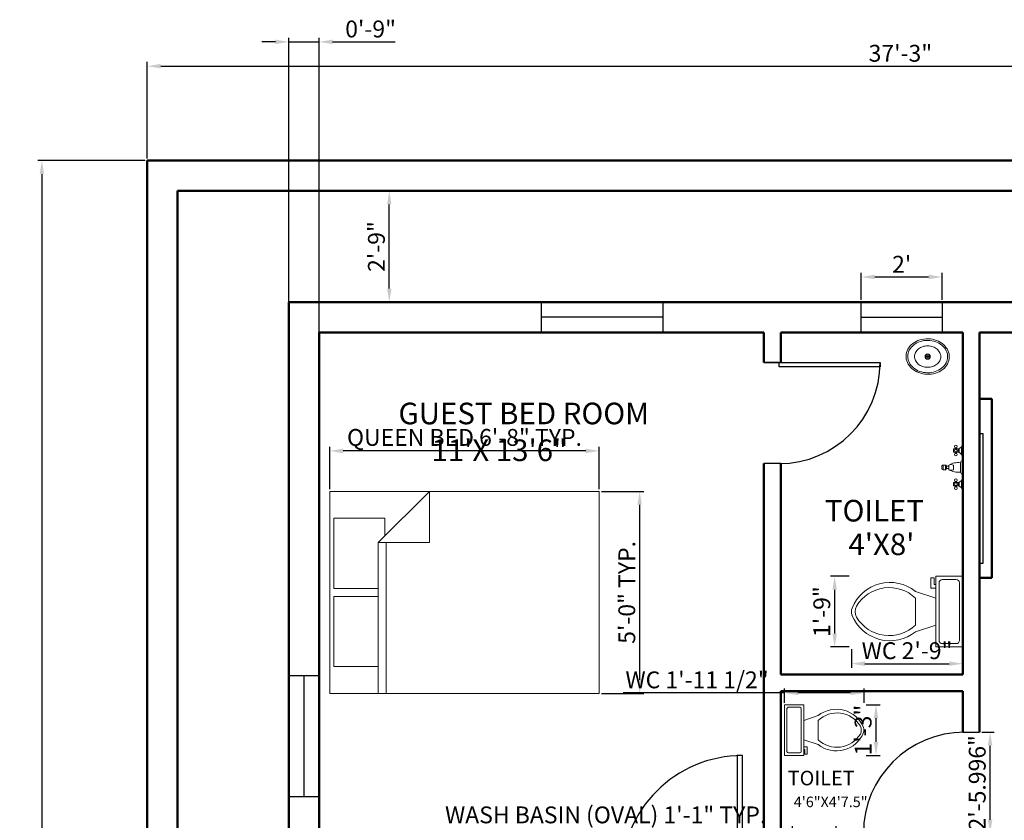
# Model space of a CAD drawing. Units: inches. Extents: x 116541 to 117938, y 135634 to 136328.
# Tile 3 of 9: x 116545 to 116838, y 136091 to 136328. Entities that reach past the tile are written whole.
import ezdxf

# ---------------------------------------------------------------- set-up
doc = ezdxf.new("R2010")
doc.units = ezdxf.units.IN
for name, color, linetype, lineweight in [('A-ANNO-DIMS', 2, 'Continuous', 18), ('A-AREA-IDEN', 3, 'Continuous', 25), ('A-DOOR', 4, 'Continuous', 25), ('A-FLOR-FIXT', 9, 'Continuous', 18), ('A-FURN', 8, 'Continuous', 18), ('A-GLAZ', 1, 'Continuous', 25), ('A-WALL', 7, 'Continuous', 50)]:
    doc.layers.add(name, color=color, linetype=linetype, lineweight=lineweight)
doc.styles.get("Standard").update_dxf_attribs({"font": 'arial.ttf'})
doc.dimstyles.new('ISO-25', dxfattribs={"dimtxt": 5, "dimasz": 4, "dimexe": 1.25, "dimexo": 0.625, "dimtad": 1, "dimdec": 3, "dimlunit": 3, "dimtxsty": 'Standard', "dimcen": 2.5, "dimadec": 0, "dimazin": 0, "dimtfac": 1, "dimtdec": 3, "dimtmove": 0, "dimatfit": 3, "dimfxl": 1, "dimarcsym": 0})

# ---------------------------------------------------------------- blocks, each defined once
blk = doc.blocks.new('*U3')
for p, q in [((0, 0), (0, -6)), ((-40, 0), (-40, -6))]:
    blk.add_line(p, q)
blk.add_lwpolyline([(0, 0), (0, 40), (-1.75, 40), (-1.75, 0)], close=True)
blk.add_arc((0, 0), 40, 90, 180)
blk = doc.blocks.new('*U2')
for p, q in [((0, 0), (0, -6)), ((40, 0), (40, -6))]:
    blk.add_line(p, q)
blk.add_lwpolyline([(0, 0), (0, 40), (1.75, 40), (1.75, 0)], close=True)
blk.add_arc((0, 0), 40, 0, 90)
blk = doc.blocks.new('Toilet - top')
for p, q in [((9.5, -6), (9.5, -2)), ((-10, -8.5), (-8, -8.5)), ((-10, -9.5), (-10, -8.5)), ((-8, -8.5), (-8, -8)), ((-7, -8), (-7, -9.5)), ((-4, -8), (-6, -14)), ((4, -8), (6, -14)), ((-7, -9.5), (-10, -9.5)), ((4, -14), (-4, -14))]:
    blk.add_line(p, q)
blk.add_lwpolyline([(10.5, -8), (10.5, 0), (-10.5, 0), (-10.5, -8)], close=True)
for points in [[(-9.5, -2), (-9.5, -6)], [(8.5, -1), (-8.5, -1)], [(-8.5, -7), (8.5, -7)]]:
    blk.add_lwpolyline(points)
for centre, radius, start, end in [((-8.62, -1.88), 0.884, 81.8699, 188.1301), ((8.62, -1.88), 0.884, 351.8699, 98.1301), ((-8.62, -6.12), 0.884, 171.8699, 278.1301), ((8.62, -6.12), 0.884, 261.8699, 8.1301), ((3.52, -21.58), 12.17, 141.4691, 247.9714), ((4.2, -21.82), 11.33, 136.3677, 238.9468), ((-3.52, -21.58), 12.17, 292.0284, 38.5307), ((-4.2, -21.82), 11.33, 301.053, 43.6321), ((0, -27.88), 4, 245.7318, 294.2682), ((0, -29), 4, 254.8605, 285.1395)]:
    blk.add_arc(centre, radius, start, end)
blk = doc.blocks.new('Faucet - Bathroom front')
for p, q in [((-0.5, 4.25), (0.5, 4.25)), ((0.5, 3.75), (-0.5, 3.75)), ((-0.5, 3), (0.5, 3)), ((-0.25, 3), (-0.25, 3.5)), ((0.25, 3.5), (0.25, 3)), ((-5, 0), (-2.25, 0)), ((-4.5087, 0.25), (-2.7408, 0.25)), ((-4, 1.625), (-4.25, 1.625)), ((-4, 1.375), (-4.25, 1.375)), ((-3.1442, 0.75), (-4.0979, 0.75)), ((-3.25, 1.625), (-3, 1.625)), ((-3.25, 1.375), (-3, 1.375)), ((-1.5, 0), (1.5, 0)), ((-1, 0.5), (1, 0.5)), ((0.5, 2), (-0.5, 2)), ((2.25, 0), (5, 0)), ((2.7413, 0.25), (4.5092, 0.25)), ((3.25, 1.625), (3, 1.625)), ((3.25, 1.375), (3, 1.375)), ((4.1058, 0.75), (3.1521, 0.75)), ((4, 1.625), (4.25, 1.625)), ((4, 1.375), (4.25, 1.375))]:
    blk.add_line(p, q)
for points in [[(-0.5, 3.75), (-0.5, 4.25)], [(-0.25, 4.5), (0.25, 4.5)], [(0.5, 4.25), (0.5, 3.75)], [(0.25, 3.5), (-0.25, 3.5)]]:
    blk.add_lwpolyline(points)
for points in [[(-4, 1), (-4, 2), (-3.25, 2), (-3.25, 1)], [(3.25, 1), (3.25, 2), (4, 2), (4, 1)]]:
    blk.add_lwpolyline(points, close=True)
for centre in [(-4.5, 1.5), (-3.625, 1.5), (-2.75, 1.5), (2.75, 1.5), (3.625, 1.5), (4.5, 1.5)]:
    blk.add_circle(centre, 0.2795)
for centre, radius, start, end in [((-0.2575, 4.2575), 0.2426, 88.22243, 181.7776), ((0.2575, 4.2575), 0.2426, 358.2224, 91.77757), ((3, 1), 4.0311, 150.2551, 187.125), ((0.6413, 2.5), 1.246, 156.3417, 203.6583), ((-0.2575, 3.7425), 0.2426, 178.2224, 271.7776), ((0.2575, 3.7425), 0.2426, 268.2224, 1.777565), ((-3, 1), 4.0311, 352.875, 29.74488), ((-0.6413, 2.5), 1.246, 336.3417, 23.65835), ((-5.375, 1.375), 1.4252, 285.2551, 344.7449), ((-1.875, 1.375), 1.4252, 195.2551, 254.7449), ((-0.7962, -0.2038), 0.7327, 106.1502, 163.8498), ((0.7962, -0.2038), 0.7327, 16.1502, 73.84979), ((1.875, 1.375), 1.4252, 285.2551, 344.7449), ((5.375, 1.375), 1.4252, 195.2551, 254.7449)]:
    blk.add_arc(centre, radius, start, end)
blk = doc.blocks.new('Bed - Queen')
for p, q in [((0, -80.00003), (0, 0)), ((0, 0), (59.99999, 0)), ((59.99999, 0), (59.99999, -80.00003)), ((7.99999, -1.2), (28.79998, -1.2)), ((7.99999, -14.4), (7.99999, -1.2)), ((28.79998, -1.2), (28.79998, -14.4)), ((31.19999, -1.2), (51.99999, -1.2)), ((31.19999, -14.4), (31.19999, -1.2)), ((51.99999, -1.2), (51.99999, -16.4)), ((0, -14.4), (44.8, -14.4)), ((59.99999, -29.6), (44.8, -14.4)), ((44.8, -14.4), (44.8, -29.6)), ((44.8, -16.8), (0, -16.8)), ((51.99999, -16.4), (46.79936, -16.4)), ((44.8, -29.6), (59.99999, -29.6)), ((59.99999, -80.00003), (0, -80.00003))]:
    blk.add_line(p, q)
blk = doc.blocks.new('Sink - Oval top')
for p, q in [((-1, 0), (1, 0)), ((0, 1), (0, -1))]:
    blk.add_line(p, q)
for points in [[(-12.23, 0.39, 0.117634), (-11.46, -3.36, 0.104469), (-8.88, -6.8, 0.090016), (-5.08, -9.07, 0.08192), (-0.32, -10.02, 0.08192), (4.49, -9.38, 0.090016), (8.42, -7.36, 0.104469), (11.22, -4.09, 0.117634), (12.23, -0.39, 0.117634), (11.46, 3.36, 0.104469), (8.88, 6.8, 0.090016), (5.08, 9.07, 0.08192), (0.32, 10.02, 0.08192), (-4.49, 9.38, 0.090016), (-8.42, 7.36, 0.104469), (-11.22, 4.09, 0.117634)], [(-11.29, 0.16, 0.118622), (-10.52, -3.25, 0.104678), (-8.07, -6.36, 0.089562), (-4.54, -8.37, 0.081185), (-0.13, -9.15, 0.081185), (4.3, -8.49, 0.089562), (7.89, -6.58, 0.104678), (10.42, -3.55, 0.118622), (11.29, -0.16, 0.118622), (10.52, 3.25, 0.104678), (8.07, 6.36, 0.089562), (4.54, 8.37, 0.081185), (0.13, 9.15, 0.081185), (-4.3, 8.49, 0.089562), (-7.89, 6.58, 0.104678), (-10.42, 3.55, 0.118622)], [(-7.42, 0.08, 0.118283), (-6.91, -2.17, 0.104607), (-5.29, -4.21, 0.089718), (-2.97, -5.53, 0.081436), (-0.07, -6.04, 0.081436), (2.84, -5.59, 0.089718), (5.2, -4.33, 0.104607), (6.86, -2.32, 0.118283), (7.42, -0.08, 0.118283), (6.91, 2.17, 0.104607), (5.29, 4.21, 0.089718), (2.97, 5.53, 0.081436), (0.07, 6.04, 0.081436), (-2.84, 5.59, 0.089718), (-5.2, 4.33, 0.104607), (-6.86, 2.32, 0.118283)]]:
    blk.add_lwpolyline(points, format="xyb", close=True)
for radius in [1.5, 1]:
    blk.add_circle((0, 0), radius)
blk = doc.blocks.new('*D26')
at = {"layer": 'A-ANNO-DIMS', "color": 0, "lineweight": -2, "transparency": 16777216}
for p, q in [((116582.55, 136286.5), (116550.65, 136286.5)), ((116551.9, 136282.5), (116551.9, 135738.5)), ((116582.55, 135734.5), (116550.65, 135734.5))]:
    blk.add_line(p, q, dxfattribs=at)
at = {"layer": 'A-ANNO-DIMS', "color": 0, "transparency": 16777216}
for points in [[(116551.23, 136282.5), (116552.56, 136282.5), (116551.9, 136286.5)], [(116551.23, 135738.5), (116552.56, 135738.5), (116551.9, 135734.5)]]:
    blk.add_solid(points, dxfattribs=at)
at = {"layer": 'Defpoints', "color": 0, "transparency": 16777216}
for p in [(116583.18, 136286.5), (116551.9, 135734.5), (116583.18, 135734.5)]:
    blk.add_point(p, dxfattribs=at)
at = {"layer": 'A-ANNO-DIMS', "color": 0, "transparency": 16777216, "insert": (116548.72, 136010.5), "char_height": 5, "attachment_point": 5, "rotation": 90}
blk.add_mtext("46'", dxfattribs=at)
blk = doc.blocks.new('*D27')
at = {"layer": 'A-ANNO-DIMS', "color": 0, "lineweight": -2, "transparency": 16777216}
for p, q in [((116583.18, 136287.13), (116583.18, 136315.79)), ((117030.18, 136287.13), (117030.18, 136315.79)), ((116587.18, 136314.54), (117026.18, 136314.54))]:
    blk.add_line(p, q, dxfattribs=at)
at = {"layer": 'A-ANNO-DIMS', "color": 0, "transparency": 16777216}
for points in [[(116587.18, 136315.21), (116587.18, 136313.88), (116583.18, 136314.54)], [(117026.18, 136315.21), (117026.18, 136313.88), (117030.18, 136314.54)]]:
    blk.add_solid(points, dxfattribs=at)
at = {"layer": 'Defpoints', "color": 0, "transparency": 16777216}
for p in [(117030.18, 136314.54), (116583.18, 136286.5), (117030.18, 136286.5)]:
    blk.add_point(p, dxfattribs=at)
at = {"layer": 'A-ANNO-DIMS', "color": 0, "transparency": 16777216, "insert": (116806.68, 136317.72), "char_height": 5, "attachment_point": 5}
blk.add_mtext('37\'-3"', dxfattribs=at)
blk = doc.blocks.new('*D29')
at = {"layer": 'A-ANNO-DIMS', "color": 0, "lineweight": -2, "transparency": 16777216}
for p, q in [((116830.8, 136116.82), (116834.55, 136116.82)), ((116833.3, 136090.82), (116833.3, 136112.82)), ((116830.8, 136086.82), (116834.55, 136086.82))]:
    blk.add_line(p, q, dxfattribs=at)
at = {"layer": 'A-ANNO-DIMS', "color": 0, "transparency": 16777216}
for points in [[(116832.63, 136112.82), (116833.97, 136112.82), (116833.3, 136116.82)], [(116832.63, 136090.82), (116833.97, 136090.82), (116833.3, 136086.82)]]:
    blk.add_solid(points, dxfattribs=at)
at = {"layer": 'Defpoints', "color": 0, "transparency": 16777216}
for p in [(116830.18, 136116.82), (116833.3, 136116.82), (116830.18, 136086.82)]:
    blk.add_point(p, dxfattribs=at)
at = {"layer": 'A-ANNO-DIMS', "color": 0, "transparency": 16777216, "insert": (116830.12, 136101.82), "char_height": 5, "attachment_point": 5, "rotation": 90}
blk.add_mtext('2\'-5.996"', dxfattribs=at)
blk = doc.blocks.new('*D32')
at = {"layer": 'A-ANNO-DIMS', "color": 0, "lineweight": -2, "transparency": 16777216}
for p, q in [((116655.62, 136277.5), (116656.25, 136277.5)), ((116655, 136248.5), (116655, 136273.5)), ((116655.62, 136244.5), (116656.25, 136244.5))]:
    blk.add_line(p, q, dxfattribs=at)
at = {"layer": 'A-ANNO-DIMS', "color": 0, "transparency": 16777216}
for points in [[(116654.33, 136273.5), (116655.66, 136273.5), (116655, 136277.5)], [(116654.33, 136248.5), (116655.66, 136248.5), (116655, 136244.5)]]:
    blk.add_solid(points, dxfattribs=at)
at = {"layer": 'Defpoints', "color": 0, "transparency": 16777216}
for p in [(116655, 136277.5), (116655, 136277.5), (116655, 136244.5)]:
    blk.add_point(p, dxfattribs=at)
at = {"layer": 'A-ANNO-DIMS', "color": 0, "transparency": 16777216, "insert": (116651.82, 136261), "char_height": 5, "attachment_point": 5, "rotation": 90}
blk.add_mtext('2\'-9"', dxfattribs=at)
blk = doc.blocks.new('*D34')
at = {"layer": 'A-ANNO-DIMS', "color": 0, "lineweight": -2, "transparency": 16777216}
for p, q in [((116795.06, 136245.13), (116795.06, 136253.21)), ((116799.06, 136251.96), (116815.06, 136251.96)), ((116819.06, 136245.13), (116819.06, 136253.21))]:
    blk.add_line(p, q, dxfattribs=at)
at = {"layer": 'A-ANNO-DIMS', "color": 0, "transparency": 16777216}
for points in [[(116799.06, 136252.63), (116799.06, 136251.29), (116795.06, 136251.96)], [(116815.06, 136252.63), (116815.06, 136251.29), (116819.06, 136251.96)]]:
    blk.add_solid(points, dxfattribs=at)
at = {"layer": 'Defpoints', "color": 0, "transparency": 16777216}
for p in [(116819.06, 136251.96), (116795.06, 136244.5), (116819.06, 136244.5)]:
    blk.add_point(p, dxfattribs=at)
at = {"layer": 'A-ANNO-DIMS', "color": 0, "transparency": 16777216, "insert": (116807.06, 136255.09), "char_height": 5, "attachment_point": 5}
blk.add_mtext("2'", dxfattribs=at)
blk = doc.blocks.new('*D62')
at = {"layer": 'A-ANNO-DIMS', "color": 0, "lineweight": -2, "transparency": 16777216}
for p, q in [((116774.69, 136086.42), (116774.69, 136088.98)), ((116787.59, 136086.42), (116787.59, 136088.98)), ((116774.69, 136087.73), (116667.73, 136087.73)), ((116783.59, 136087.73), (116778.69, 136087.73))]:
    blk.add_line(p, q, dxfattribs=at)
at = {"layer": 'A-ANNO-DIMS', "color": 0, "transparency": 16777216}
for points in [[(116778.69, 136088.4), (116778.69, 136087.07), (116774.69, 136087.73)], [(116783.59, 136088.4), (116783.59, 136087.07), (116787.59, 136087.73)]]:
    blk.add_solid(points, dxfattribs=at)
at = {"layer": 'Defpoints', "color": 0, "transparency": 16777216}
for p in [(116774.69, 136087.73), (116774.69, 136085.8), (116787.59, 136085.8)]:
    blk.add_point(p, dxfattribs=at)
at = {"layer": 'A-ANNO-DIMS', "color": 0, "transparency": 16777216, "insert": (116719.21, 136091.64), "char_height": 5, "attachment_point": 5}
blk.add_mtext('WASH BASIN (OVAL) 1\'-1" TYP.', dxfattribs=at)
blk = doc.blocks.new('*D70')
at = {"layer": 'A-ANNO-DIMS', "color": 0, "lineweight": -2, "transparency": 16777216}
for p, q in [((116637.31, 136188.95), (116637.31, 136201.58)), ((116713.31, 136200.33), (116641.31, 136200.33)), ((116717.31, 136188.95), (116717.31, 136201.58))]:
    blk.add_line(p, q, dxfattribs=at)
at = {"layer": 'A-ANNO-DIMS', "color": 0, "transparency": 16777216}
for points in [[(116641.31, 136200.99), (116641.31, 136199.66), (116637.31, 136200.33)], [(116713.31, 136200.99), (116713.31, 136199.66), (116717.31, 136200.33)]]:
    blk.add_solid(points, dxfattribs=at)
at = {"layer": 'Defpoints', "color": 0, "transparency": 16777216}
for p in [(116637.31, 136200.33), (116637.31, 136188.33), (116717.31, 136188.33)]:
    blk.add_point(p, dxfattribs=at)
at = {"layer": 'A-ANNO-DIMS', "color": 0, "transparency": 16777216, "insert": (116677.31, 136203.69), "char_height": 5, "attachment_point": 5}
blk.add_mtext('QUEEN BED 6\'-8" TYP.', dxfattribs=at)
blk = doc.blocks.new('*D71')
at = {"layer": 'A-ANNO-DIMS', "color": 0, "lineweight": -2, "transparency": 16777216}
for p, q in [((116717.93, 136188.33), (116730.56, 136188.33)), ((116729.31, 136132.33), (116729.31, 136184.33)), ((116717.93, 136128.33), (116730.56, 136128.33))]:
    blk.add_line(p, q, dxfattribs=at)
at = {"layer": 'A-ANNO-DIMS', "color": 0, "transparency": 16777216}
for points in [[(116728.64, 136184.33), (116729.97, 136184.33), (116729.31, 136188.33)], [(116728.64, 136132.33), (116729.97, 136132.33), (116729.31, 136128.33)]]:
    blk.add_solid(points, dxfattribs=at)
at = {"layer": 'Defpoints', "color": 0, "transparency": 16777216}
for p in [(116717.31, 136188.33), (116729.31, 136188.33), (116717.31, 136128.33)]:
    blk.add_point(p, dxfattribs=at)
at = {"layer": 'A-ANNO-DIMS', "color": 0, "transparency": 16777216, "insert": (116726.13, 136158.33), "char_height": 5, "attachment_point": 5, "rotation": 90}
blk.add_mtext('5\'-0" TYP.', dxfattribs=at)
blk = doc.blocks.new('*D74')
at = {"layer": 'A-ANNO-DIMS', "color": 0, "lineweight": -2, "transparency": 16777216}
for p, q in [((116772.26, 136125.59), (116772.26, 136129.76)), ((116795.89, 136125.59), (116795.89, 136129.76)), ((116772.26, 136128.51), (116724.4, 136128.51)), ((116791.89, 136128.51), (116776.26, 136128.51))]:
    blk.add_line(p, q, dxfattribs=at)
at = {"layer": 'A-ANNO-DIMS', "color": 0, "transparency": 16777216}
for points in [[(116776.26, 136129.18), (116776.26, 136127.84), (116772.26, 136128.51)], [(116791.89, 136129.18), (116791.89, 136127.84), (116795.89, 136128.51)]]:
    blk.add_solid(points, dxfattribs=at)
at = {"layer": 'Defpoints', "color": 0, "transparency": 16777216}
for p in [(116772.26, 136128.51), (116772.26, 136124.97), (116795.89, 136124.97)]:
    blk.add_point(p, dxfattribs=at)
at = {"layer": 'A-ANNO-DIMS', "color": 0, "transparency": 16777216, "insert": (116746.33, 136131.72), "char_height": 5, "attachment_point": 5}
blk.add_mtext('WC 1\'-11 1/2"', dxfattribs=at)
blk = doc.blocks.new('*D75')
at = {"layer": 'A-ANNO-DIMS', "color": 0, "lineweight": -2, "transparency": 16777216}
for p, q in [((116796.52, 136124.97), (116800.69, 136124.97)), ((116799.44, 136113.95), (116799.44, 136120.97)), ((116796.52, 136109.95), (116800.69, 136109.95))]:
    blk.add_line(p, q, dxfattribs=at)
at = {"layer": 'A-ANNO-DIMS', "color": 0, "transparency": 16777216}
for points in [[(116798.77, 136120.97), (116800.1, 136120.97), (116799.44, 136124.97)], [(116798.77, 136113.95), (116800.1, 136113.95), (116799.44, 136109.95)]]:
    blk.add_solid(points, dxfattribs=at)
at = {"layer": 'Defpoints', "color": 0, "transparency": 16777216}
for p in [(116795.89, 136124.97), (116799.44, 136124.97), (116795.89, 136109.95)]:
    blk.add_point(p, dxfattribs=at)
at = {"layer": 'A-ANNO-DIMS', "color": 0, "transparency": 16777216, "insert": (116796.26, 136117.46), "char_height": 5, "attachment_point": 5, "rotation": 90}
blk.add_mtext('1\'-3"', dxfattribs=at)
blk = doc.blocks.new('*D76')
at = {"layer": 'A-ANNO-DIMS', "color": 0, "lineweight": -2, "transparency": 16777216}
for p, q in [((116792.13, 136141.5), (116792.13, 136135.92)), ((116825.18, 136141.5), (116825.18, 136135.92)), ((116796.13, 136137.17), (116821.18, 136137.17))]:
    blk.add_line(p, q, dxfattribs=at)
at = {"layer": 'A-ANNO-DIMS', "color": 0, "transparency": 16777216}
for points in [[(116796.13, 136137.84), (116796.13, 136136.5), (116792.13, 136137.17)], [(116821.18, 136137.84), (116821.18, 136136.5), (116825.18, 136137.17)]]:
    blk.add_solid(points, dxfattribs=at)
at = {"layer": 'Defpoints', "color": 0, "transparency": 16777216}
for p in [(116792.13, 136142.13), (116825.18, 136142.13), (116825.18, 136137.17)]:
    blk.add_point(p, dxfattribs=at)
at = {"layer": 'A-ANNO-DIMS', "color": 0, "transparency": 16777216, "insert": (116808.65, 136140.38), "char_height": 5, "attachment_point": 5}
blk.add_mtext('WC 2\'-9"', dxfattribs=at)
blk = doc.blocks.new('*D77')
at = {"layer": 'A-ANNO-DIMS', "color": 0, "lineweight": -2, "transparency": 16777216}
for p, q in [((116791.51, 136163.13), (116785.92, 136163.13)), ((116787.17, 136159.13), (116787.17, 136146.13)), ((116791.51, 136142.13), (116785.92, 136142.13))]:
    blk.add_line(p, q, dxfattribs=at)
at = {"layer": 'A-ANNO-DIMS', "color": 0, "transparency": 16777216}
for points in [[(116786.51, 136159.13), (116787.84, 136159.13), (116787.17, 136163.13)], [(116786.51, 136146.13), (116787.84, 136146.13), (116787.17, 136142.13)]]:
    blk.add_solid(points, dxfattribs=at)
at = {"layer": 'Defpoints', "color": 0, "transparency": 16777216}
for p in [(116792.13, 136163.13), (116787.17, 136142.13), (116792.13, 136142.13)]:
    blk.add_point(p, dxfattribs=at)
at = {"layer": 'A-ANNO-DIMS', "color": 0, "transparency": 16777216, "insert": (116784, 136152.63), "char_height": 5, "attachment_point": 5, "rotation": 90}
blk.add_mtext('1\'-9"', dxfattribs=at)
blk = doc.blocks.new('*D105')
at = {"layer": 'A-ANNO-DIMS', "color": 0, "lineweight": -2, "transparency": 16777216}
for p, q in [((116621.18, 136321.75), (116617.18, 136321.75)), ((116625.18, 136098.24), (116625.18, 136323)), ((116625.18, 136321.75), (116634.18, 136321.75)), ((116634.18, 136098.24), (116634.18, 136323)), ((116638.18, 136321.75), (116656.72, 136321.75))]:
    blk.add_line(p, q, dxfattribs=at)
at = {"layer": 'A-ANNO-DIMS', "color": 0, "transparency": 16777216}
for points in [[(116621.18, 136322.42), (116621.18, 136321.09), (116625.18, 136321.75)], [(116638.18, 136322.42), (116638.18, 136321.09), (116634.18, 136321.75)]]:
    blk.add_solid(points, dxfattribs=at)
at = {"layer": 'Defpoints', "color": 0, "transparency": 16777216}
for p in [(116634.18, 136321.75), (116625.18, 136097.62), (116634.18, 136097.62)]:
    blk.add_point(p, dxfattribs=at)
at = {"layer": 'A-ANNO-DIMS', "color": 0, "transparency": 16777216, "insert": (116649.45, 136324.93), "char_height": 5, "attachment_point": 5}
blk.add_mtext('0\'-9"', dxfattribs=at)

msp = doc.modelspace()

# ---------------------------------------------------------------- linework, layer by layer
at = {"layer": 'A-DOOR'}
for points in [[(116766.1763, 136226.5704), (116771.1763, 136226.5704)], [(116771.1763, 136196.5704), (116766.1763, 136196.5704)], [(116825.1763, 136116.8229), (116830.1763, 136116.8229)]]:
    msp.add_lwpolyline(points, dxfattribs=at)
at = {"layer": 'A-GLAZ'}
for p, q in [((116736.1763, 136240.0034), (116700.1763, 136240.0034)), ((116795.057, 136240.0034), (116819.057, 136240.0034)), ((116830.1763, 136205.5237), (116831.1731, 136205.5237)), ((116831.1731, 136205.5237), (116831.1731, 136166.9453)), ((116831.1731, 136166.9453), (116830.1763, 136166.9453)), ((116629.6763, 136133.6191), (116629.6763, 136097.6191))]:
    msp.add_line(p, q, dxfattribs=at)
for points in [[(116736.1763, 136244.5034), (116736.1763, 136235.5034), (116700.1763, 136235.5034), (116700.1763, 136244.5034)], [(116795.057, 136235.5034), (116795.057, 136244.5034), (116819.057, 136244.5034), (116819.057, 136235.5034)], [(116625.1763, 136133.6191), (116634.1763, 136133.6191), (116634.1763, 136097.6191), (116625.1763, 136097.6191)]]:
    msp.add_lwpolyline(points, close=True, dxfattribs=at)
at = {"layer": 'A-WALL'}
for p, q in [((116583.1763, 136286.5034), (117000.1763, 136286.5034)), ((116583.1763, 136286.5034), (116583.1763, 135734.5034)), ((116592.1763, 136277.5034), (117000.1763, 136277.5034)), ((116592.1763, 136277.5034), (116592.1763, 135743.5034)), ((116625.1763, 136244.5034), (116982.7496, 136244.5034)), ((116625.1763, 136244.5034), (116625.1763, 135950.5034)), ((116634.1763, 136235.5034), (116766.1763, 136235.5034)), ((116634.1763, 136235.5034), (116634.1763, 135950.5034)), ((116766.1763, 136235.5034), (116766.1763, 136226.5704)), ((116771.1763, 136235.5034), (116771.1763, 136226.5704)), ((116771.1763, 136235.5034), (116825.1763, 136235.5034)), ((116825.1763, 136235.5034), (116825.1763, 136134.0034)), ((116830.1763, 136235.5034), (116830.1763, 136116.8229)), ((116830.1763, 136235.5034), (116973.7496, 136235.5034)), ((116830.1763, 136215.7448), (116833.8106, 136215.7448)), ((116833.8106, 136215.7448), (116833.8106, 136162.6837)), ((116766.1763, 136196.5704), (116766.1763, 136073.5034)), ((116771.1763, 136196.5704), (116771.1763, 136134.0034)), ((116833.8106, 136162.6837), (116830.1763, 136162.6837)), ((116771.1763, 136134.0034), (116825.1763, 136134.0034)), ((116771.1763, 136129.0034), (116825.1763, 136129.0034)), ((116771.1763, 136129.0034), (116771.1763, 136073.5034)), ((116825.1763, 136129.0034), (116825.1763, 136116.8229))]:
    msp.add_line(p, q, dxfattribs=at)

# ---------------------------------------------------------------- block references
at = {"layer": 'A-DOOR'}
for p, xscale, yscale, zscale, rotation in [((116770.6763, 136226.5704), 0.75, 0.75, 0.75, 270), ((116825.6769, 136086.8229), 0.749895633020561, 0.749895633020561, 0.749895633020561, 90)]:
    msp.add_blockref('*U2', p, dxfattribs=dict(at, xscale=xscale, yscale=yscale, zscale=zscale, rotation=rotation))
at = {"layer": 'A-DOOR', "xscale": 0.9, "yscale": 0.9, "zscale": 0.9}
msp.add_blockref('*U3', (116759.8277, 136073.9034), dxfattribs=at)
at = {"layer": 'A-FLOR-FIXT'}
for name, p, xscale, yscale, zscale, rotation in [('Sink - Oval top', (116814.7727, 136228.3379), 0.5252454991663538, 0.5252454991663538, 0.5252454991663538, 180), ('Faucet - Bathroom front', (116825.1763, 136195.4396), 1.375236022188706, 1.375236022188706, 1.375236022188706, 90), ('Toilet - top', (116772.2572, 136117.4564), 0.7151778874048526, 0.7151778874048526, 0.7151778874048526, 89.99999999999999)]:
    msp.add_blockref(name, p, dxfattribs=dict(at, xscale=xscale, yscale=yscale, zscale=zscale, rotation=rotation))
at = {"layer": 'A-FLOR-FIXT', "rotation": 270}
msp.add_blockref('Toilet - top', (116825.1763, 136152.6285), dxfattribs=at)
at = {"layer": 'A-FURN', "rotation": 90}
msp.add_blockref('Bed - Queen', (116637.3079, 136128.3258), dxfattribs=at)

# ---------------------------------------------------------------- texts
at = {"layer": 'A-AREA-IDEN'}
for s, height, p in [('GUEST BED ROOM', 6.408368, (116657.7191, 136208.2362)), ('     11\'X 13\'6"', 6.408368, (116657.7191, 136197.3136)), ('TOILET', 6.40837, (116784.2693, 136179.3804)), ("4'X8'", 6.40837, (116791.2572, 136169.4064)), ('TOILET', 4.32687, (116773.2314, 136101.0568)), ('4\'6"X4\'7.5"', 3.126205, (116775.0501, 136094.5839))]:
    msp.add_text(s, height=height, dxfattribs=at).set_placement(p)

# ---------------------------------------------------------------- dimensions: what is measured, and where the dimension line sits
at = {"layer": 'A-ANNO-DIMS'}
for base, p1, p2, override, picture, middle in [((116634.1763, 136321.7534), (116625.1763, 136097.6191), (116634.1763, 136097.6191), {"dimdec": 1, "dimlfac": 1, "dimrnd": 0, "dimzin": 1, "dimdsep": 46, "dimlunit": 4, "dimfrac": 2}, '*D105', (116649.4469, 136324.9313)), ((117030.1763, 136314.5423), (116583.1763, 136286.5034), (117030.1763, 136286.5034), {"dimclrd": 0, "dimclre": 0, "dimclrt": 0}, '*D27', (116806.6763, 136317.7219)), ((116819.057, 136251.9593), (116795.057, 136244.5034), (116819.057, 136244.5034), {"dimclrd": 0, "dimclre": 0, "dimclrt": 0}, '*D34', (116807.057, 136255.0945))]:
    dim = msp.add_linear_dim(base=base, p1=p1, p2=p2, dimstyle='ISO-25', override=override, dxfattribs=at)
    dim.commit()
    dim.dimension.update_dxf_attribs({"geometry": picture, "text_midpoint": middle})
for base, p1, p2, angle, override, picture, middle in [((116551.8967, 135734.5034), (116583.1763, 136286.5034), (116583.1763, 135734.5034), 90, {"dimclrd": 0, "dimclre": 0, "dimclrt": 0}, '*D26', (116548.7188, 136010.5034)), ((116654.9967, 136277.5034), (116654.9967, 136244.5034), (116654.9967, 136277.5034), 90, {"dimclrd": 0, "dimclre": 0, "dimclrt": 0}, '*D32', (116651.8188, 136261.0034)), ((116787.1731, 136142.1285), (116792.13, 136163.1285), (116792.13, 136142.1285), 270, {"dimdec": 1, "dimrnd": 0, "dimzin": 1, "dimlunit": 4, "dimfrac": 2}, '*D77', (116783.9952, 136152.6285)), ((116799.4362, 136124.9657), (116795.8911, 136109.947), (116795.8911, 136124.9657), 90, {"dimdec": 1, "dimrnd": 0, "dimzin": 1, "dimlunit": 4, "dimfrac": 2}, '*D75', (116796.2566, 136117.4564)), ((116833.2999, 136116.8187), (116830.1763, 136086.8229), (116830.1763, 136116.8187), 90, {"dimclrd": 0, "dimclre": 0, "dimclrt": 0}, '*D29', (116830.1221, 136101.8208))]:
    dim = msp.add_linear_dim(base=base, p1=p1, p2=p2, angle=angle, dimstyle='ISO-25', override=override, dxfattribs=at)
    dim.commit()
    dim.dimension.update_dxf_attribs({"geometry": picture, "text_midpoint": middle})
for base, p1, p2, angle, text, picture, middle in [((116637.3079, 136200.3258), (116717.3079, 136188.3258), (116637.3079, 136188.3258), 180, 'QUEEN BED <> TYP.', '*D70', (116677.3079, 136203.6895)), ((116729.3079, 136188.3258), (116717.3079, 136128.3258), (116717.3079, 136188.3258), 90, '<> TYP.', '*D71', (116726.1301, 136158.3258)), ((116772.2572, 136128.5108), (116795.8911, 136124.9657), (116772.2572, 136124.9657), 180, 'WC <>', '*D74', (116746.3276, 136131.7211)), ((116774.6928, 136087.7343), (116787.588, 136085.8), (116774.6928, 136085.8), 180, 'WASH BASIN (OVAL) <> TYP.', '*D62', (116719.2134, 136091.6386))]:
    dim = msp.add_linear_dim(base=base, p1=p1, p2=p2, angle=angle, text=text, dimstyle='ISO-25', override={"dimdec": 1, "dimrnd": 0, "dimzin": 1, "dimlunit": 4, "dimfrac": 2}, dxfattribs=at)
    dim.commit()
    dim.dimension.update_dxf_attribs({"geometry": picture, "text_midpoint": middle})
dim = msp.add_linear_dim(base=(116825.1763, 136137.1716), p1=(116792.13, 136142.1285), p2=(116825.1763, 136142.1285), text='WC <>', dimstyle='ISO-25', override={"dimdec": 1, "dimrnd": 0, "dimzin": 1, "dimlunit": 4, "dimfrac": 2}, dxfattribs=at)
dim.commit()
dim.dimension.update_dxf_attribs({"geometry": '*D76', "text_midpoint": (116808.6531, 136140.3819)})

doc.saveas('drawing.dxf')
